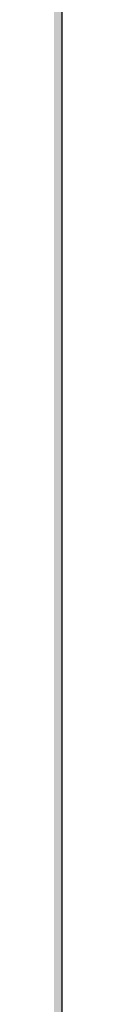
# Model space of a CAD drawing. Units: inches. Extents: x 2091 to 2899, y 967 to 2217.
# Tile 61 of 256: x 2212.1436 to 2212.1443, y 1099.9988 to 1100.1654. Entities that reach past the tile are written whole.
import ezdxf

# ---------------------------------------------------------------- set-up
doc = ezdxf.new("R2010")
doc.units = ezdxf.units.IN
doc.layers.add('A-ANNO-DIMS', color=2, linetype='Continuous', lineweight=18)
doc.layers.add('A-WALL-PATT', color=141, linetype='Continuous', lineweight=13, true_color=0xadddf7)
doc.styles.get("Standard").update_dxf_attribs({"font": 'arial.ttf'})
doc.dimstyles.new('ISO-25', dxfattribs={"dimtxt": 4, "dimasz": 4, "dimexe": 1.25, "dimexo": 0.625, "dimtad": 1, "dimdec": 0, "dimlunit": 3, "dimtxsty": 'Standard', "dimcen": 2.5, "dimadec": 0, "dimazin": 0, "dimtfac": 1, "dimtdec": 0, "dimtmove": 0, "dimatfit": 3, "dimfxl": 1, "dimarcsym": 0})

# ---------------------------------------------------------------- blocks, each defined once
blk = doc.blocks.new('*D71')
at = {"layer": 'A-ANNO-DIMS', "color": 0, "lineweight": -2, "transparency": 16777216}
for p, q in [((2212.1436, 1351.29406), (2212.1436, 969.4643)), ((2452.1436, 1351.29406), (2452.1436, 969.4643)), ((2216.1436, 970.7143), (2448.1436, 970.7143))]:
    blk.add_line(p, q, dxfattribs=at)
at = {"layer": 'A-ANNO-DIMS', "color": 0, "transparency": 16777216}
for points in [[(2216.1436, 971.38097), (2216.1436, 970.04764), (2212.1436, 970.7143)], [(2448.1436, 971.38097), (2448.1436, 970.04764), (2452.1436, 970.7143)]]:
    blk.add_solid(points, dxfattribs=at)
at = {"layer": 'Defpoints', "color": 0, "transparency": 16777216}
for p in [(2212.1436, 1351.91906), (2452.1436, 1351.91906), (2452.1436, 970.7143)]:
    blk.add_point(p, dxfattribs=at)
at = {"layer": 'A-ANNO-DIMS', "color": 0, "transparency": 16777216, "insert": (2332.1436, 973.38159), "char_height": 4, "attachment_point": 5}
blk.add_mtext('20\'-0"', dxfattribs=at)
blk = doc.blocks.new('*D75')
at = {"layer": 'A-ANNO-DIMS', "color": 0, "lineweight": -2, "transparency": 16777216}
for p, q in [((2212.1436, 1274.79406), (2212.1436, 969.4643)), ((2308.1436, 1274.79406), (2308.1436, 969.4643)), ((2216.1436, 970.7143), (2304.1436, 970.7143))]:
    blk.add_line(p, q, dxfattribs=at)
at = {"layer": 'A-ANNO-DIMS', "color": 0, "transparency": 16777216}
for points in [[(2216.1436, 971.38097), (2216.1436, 970.04764), (2212.1436, 970.7143)], [(2304.1436, 971.38097), (2304.1436, 970.04764), (2308.1436, 970.7143)]]:
    blk.add_solid(points, dxfattribs=at)
at = {"layer": 'Defpoints', "color": 0, "transparency": 16777216}
for p in [(2212.1436, 1275.41906), (2308.1436, 1275.41906), (2308.1436, 970.7143)]:
    blk.add_point(p, dxfattribs=at)
at = {"layer": 'A-ANNO-DIMS', "color": 0, "transparency": 16777216, "insert": (2260.1436, 973.38159), "char_height": 4, "attachment_point": 5}
blk.add_mtext('8\'-0"', dxfattribs=at)
blk = doc.blocks.new('*D91')
at = {"layer": 'A-ANNO-DIMS', "color": 0, "lineweight": -2, "transparency": 16777216}
for p, q in [((2211.65063, 1152.24706), (2098.31133, 1152.24706)), ((2099.56133, 1103.91906), (2099.56133, 1148.24706)), ((2211.5186, 1099.91906), (2098.31133, 1099.91906))]:
    blk.add_line(p, q, dxfattribs=at)
at = {"layer": 'A-ANNO-DIMS', "color": 0, "transparency": 16777216}
for points in [[(2098.89467, 1148.24706), (2100.228, 1148.24706), (2099.56133, 1152.24706)], [(2098.89467, 1103.91906), (2100.228, 1103.91906), (2099.56133, 1099.91906)]]:
    blk.add_solid(points, dxfattribs=at)
at = {"layer": 'Defpoints', "color": 0, "transparency": 16777216}
for p in [(2099.56133, 1152.24706), (2212.27563, 1152.24706), (2212.1436, 1099.91906)]:
    blk.add_point(p, dxfattribs=at)
at = {"layer": 'A-ANNO-DIMS', "color": 0, "transparency": 16777216, "insert": (2096.86812, 1126.08306), "char_height": 4, "attachment_point": 5, "rotation": 90}
blk.add_mtext('4\'-4 1/2"', dxfattribs=at)

msp = doc.modelspace()

# ---------------------------------------------------------------- hatches: boundary and pattern name
at = {"layer": 'A-WALL-PATT'}
h = msp.add_hatch(color=256, dxfattribs=at)
h.dxf.hatch_style = 1
h.paths.add_polyline_path([(2803.1436, 2050.91906), (2203.1436, 2050.91906), (2203.1436, 1090.91906), (2803.1436, 1090.91906)])
h.paths.add_polyline_path([(2635.79885, 1147.54046), (2674.52405, 1147.54046, 0.376086), (2678.52967, 1152.8802), (2678.52967, 1159.55647, 0.333335), (2674.52432, 1163.56185), (2674.52432, 1163.56185), (2674.52432, 1192.93439), (2635.80597, 1192.93439), (2597.08762, 1192.93439), (2597.08762, 1163.56185, 0.333335), (2593.08228, 1159.55647), (2593.08228, 1152.8802, 0.376086), (2597.08789, 1147.54046)], flags=0)
h.paths.add_polyline_path([(2436.01043, 1278.24078, 0.000483), (2435.95264, 1278.21503, -0.001328), (2435.93563, 1278.11169, -0.001711), (2436.11644, 1278.04076, 0.002185)], flags=0)
h.paths.add_polyline_path([(2794.1436, 1143.41906), (2794.1436, 1347.41906), (2543.37017, 1347.41906), (2543.37017, 1351.91906), (2794.1436, 1351.91906), (2794.1436, 1392.71355), (2793.9474, 1392.71355), (2793.9474, 1473.5369), (2794.1436, 1473.5369), (2794.1436, 1531.91906), (2650.1436, 1531.91906), (2650.1436, 1536.41906), (2794.1436, 1536.41906), (2794.1436, 1692.41906), (2609.37561, 1692.41906), (2609.37561, 1644.41906), (2604.87561, 1644.41906), (2604.87561, 1744.91906), (2609.37561, 1744.91906), (2609.37561, 1696.91906), (2794.1436, 1696.91906), (2794.1436, 1780.91906), (2609.6436, 1780.91906), (2493.87561, 1780.91906), (2493.87561, 1785.41906), (2609.6436, 1785.41906), (2794.1436, 1785.41906), (2794.1436, 1847.93882), (2793.95122, 1847.93882), (2793.95122, 1928.76217), (2794.1436, 1928.76217), (2794.1436, 1941.41906), (2614.1436, 1941.41906), (2614.1436, 1821.41906), (2609.6436, 1821.41906), (2609.6436, 1941.41906), (2392.1436, 1941.41906), (2392.1436, 1819.91906), (2387.6436, 1819.91906), (2387.6436, 1941.41906), (2212.1436, 1941.41906), (2212.1436, 1783.91906), (2392.1436, 1783.91906), (2392.1436, 1780.91906), (2212.1436, 1780.91906), (2212.1436, 1629.41906), (2387.6436, 1629.41906), (2387.6436, 1744.91906), (2392.1436, 1744.91906), (2392.1436, 1627.91906), (2317.1436, 1627.91906), (2317.1436, 1551.41906), (2317.1436, 1536.41906), (2459.38359, 1536.41906), (2459.38359, 1602.39648), (2463.88359, 1602.39648), (2463.88359, 1531.91906), (2456.6436, 1531.91906), (2456.6436, 1529.91906), (2452.1436, 1529.91906), (2452.1436, 1531.91906), (2312.6436, 1531.91906), (2312.6436, 1551.41906), (2306.1436, 1551.41906), (2306.1436, 1555.91906), (2308.1436, 1555.91906), (2308.1436, 1551.41906), (2312.6436, 1551.41906), (2312.6436, 1627.91906), (2212.1436, 1627.91906), (2212.1436, 1555.91906), (2270.1436, 1555.91906), (2270.1436, 1551.41906), (2212.1436, 1551.41906), (2212.1436, 1351.91906), (2272.1436, 1351.91906), (2272.1436, 1347.41906), (2212.1436, 1347.41906), (2212.1436, 1275.41906), (2308.1436, 1275.41906), (2308.1436, 1351.91906), (2452.1436, 1351.91906), (2452.1436, 1493.91906), (2456.6436, 1493.91906), (2456.6436, 1347.41906), (2312.6436, 1347.41906), (2312.6436, 1270.91906), (2212.1436, 1270.91906), (2212.1436, 1099.91906), (2281.23752, 1099.91906), (2282.87104, 1110.9138), (2282.00834, 1116.9966), (2278.55774, 1121.4204), (2268.20564, 1128.0562), (2272.08764, 1128.0562), (2273.81294, 1131.927), (2279.42034, 1134.6919), (2285.02784, 1135.2449), (2287.61584, 1137.4568), (2288.04714, 1138.0098), (2289.34114, 1140.7747), (2291.06654, 1139.6687), (2292.36054, 1135.2449), (2295.37984, 1136.9038), (2296.24254, 1135.7979), (2297.10524, 1133.033), (2300.12464, 1138.0098), (2303.14394, 1138.0098), (2304.43794, 1135.7979), (2303.14394, 1133.586), (2306.59464, 1134.6919), (2307.88874, 1133.033), (2310.90804, 1135.2449), (2313.92744, 1134.1389), (2315.62686, 1132.4271), (2308.32004, 1117.5496), (2290.20384, 1109.8079), (2288.90984, 1103.1721), (2289.27231, 1099.91906), (2434.91823, 1099.91906), (2431.59323, 1124.78806), (2429.93023, 1169.55306), (2430.92718, 1240.51969), (2435.65893, 1238.18613), (2437.13523, 1196.55406), (2438.79823, 1143.97306), (2442.67823, 1111.99806), (2446.55823, 1099.91906), (2794.1436, 1099.91906), (2794.1436, 1138.91906), (2548.03245, 1138.91906), (2548.03245, 1143.41906), (2548.03245, 1148.81906), (2546.66846, 1148.03156), (2528.68569, 1179.17862, 0.256256), (2512.03245, 1148.81906), (2512.03245, 1143.41906), (2512.03245, 1138.91906), (2507.53245, 1138.91906), (2507.53245, 1143.41906), (2507.53245, 1148.81906, 0.256256), (2490.8792, 1179.17862), (2472.89644, 1148.03156), (2471.53245, 1148.81906), (2471.53245, 1143.41906), (2467.03245, 1143.41906), (2467.03245, 1269.94579, 0.039061), (2460.90999, 1273.58006), (2467.03245, 1273.58006), (2467.03245, 1286.32536, 0.014511), (2465.21619, 1286.76191), (2467.03245, 1287.05258), (2467.03245, 1323.41906), (2471.53245, 1323.41906), (2471.53245, 1148.81906), (2489.53245, 1179.99597), (2490.89644, 1179.20847), (2490.8792, 1179.17862, -0.256256), (2507.53245, 1148.81906), (2507.53245, 1143.41906), (2512.03245, 1143.41906), (2512.03245, 1148.81906, -0.256256), (2528.68569, 1179.17862), (2528.66846, 1179.20847), (2530.03245, 1179.99597), (2548.03245, 1148.81906), (2548.03245, 1143.41906)], flags=16)
h.paths.add_polyline_path([(2607.76855, 1200.94508), (2607.76855, 1265.03063), (2597.08762, 1281.05201), (2619.78459, 1281.05201), (2627.79528, 1337.12686), (2635.79885, 1337.12686), (2643.81666, 1337.12686), (2651.82736, 1281.05201), (2674.52432, 1281.05201), (2663.8434, 1265.03063), (2663.8434, 1200.94508), (2635.80597, 1200.94508)], flags=0)
edge = h.paths.add_edge_path(flags=0)
edge.add_ellipse((13303.89622, 1272.99872), major_axis=(-10595.31304, 0), ratio=0.84230387009, start_angle=0.628237219, end_angle=0.6465541, ccw=False)
edge.add_ellipse((2711.70045, 1156.85268), major_axis=(2.21977, 0), ratio=0.8423039, start_angle=111.53524, end_angle=180.62824, ccw=False)
edge.add_ellipse((13303.15629, 1272.99872), major_axis=(-10593.02631, 0), ratio=0.84230386954, start_angle=0.528271472, end_angle=0.646554097, ccw=False)
edge.add_line((2710.7646, 1175.3333), (2710.12999, 1175.3333))
edge.add_ellipse((2710.12999, 1176.57978), major_axis=(1.47985, 0), ratio=0.8423039, start_angle=180, end_angle=270, ccw=False)
edge.add_line((2708.65014, 1176.57978), (2708.65014, 1200.78291))
edge.add_ellipse((2710.12999, 1200.78291), major_axis=(1.47985, 0), ratio=0.8423039, start_angle=90, end_angle=180, ccw=False)
edge.add_line((2710.12999, 1202.02939), (2710.46508, 1202.02939))
edge.add_ellipse((13303.15629, 1272.99872), major_axis=(-10593.02631, 0), ratio=0.84230386954, start_angle=-0.090229089, end_angle=0.383866779, ccw=False)
edge.add_ellipse((2710.12999, 1290.92703), major_axis=(-1.47985, 0), ratio=0.8423039, start_angle=0, end_angle=90, ccw=False)
edge.add_line((2708.65014, 1290.92703), (2708.65014, 1315.13017))
edge.add_ellipse((2710.12999, 1315.13017), major_axis=(-1.47985, 0), ratio=0.8423039, start_angle=-90, end_angle=0, ccw=False)
edge.add_line((2710.12999, 1316.37665), (2710.70631, 1316.37665))
edge.add_ellipse((3238.40172, 1296.28957), major_axis=(528.234, 0), ratio=0.84230387, start_angle=176.3495724, end_angle=177.8200497, ccw=False)
edge.add_ellipse((2775.06304, 1071.4507), major_axis=(313.30776, 0), ratio=0.84230387, start_angle=102.1259656, end_angle=103.780529, ccw=False)
edge.add_ellipse((2775.06304, 1078.3057), major_axis=(-305.30289, 0), ratio=0.84230387, start_angle=-79.790461, end_angle=-77.5553727, ccw=False)
edge.add_ellipse((2695.14177, 1541.97538), major_axis=(-250.96022, 0), ratio=0.84230387, start_angle=99.256566, end_angle=102.5549326)
edge.add_line((2741.41033, 1334.21426), (2747.13255, 1337.37848))
edge.add_ellipse((2747.53862, 1336.85748), major_axis=(-0.73992, 0), ratio=0.842304, start_angle=270, end_angle=307.93313, ccw=False)
edge.add_ellipse((2747.53862, 1336.85748), major_axis=(-0.73992, 0), ratio=0.842304, start_angle=232.06687, end_angle=270, ccw=False)
edge.add_line((2747.94469, 1337.37848), (2753.66691, 1334.21426))
edge.add_ellipse((2799.93547, 1541.97538), major_axis=(250.96022, 0), ratio=0.84230387, start_angle=257.4450674, end_angle=260.743434)
edge.add_ellipse((2720.01419, 1078.3057), major_axis=(305.30289, 0), ratio=0.84230387, start_angle=77.5553727, end_angle=79.790461, ccw=False)
edge.add_ellipse((2720.01419, 1071.4507), major_axis=(-313.30776, 0), ratio=0.84230387, start_angle=256.219471, end_angle=257.8740344, ccw=False)
edge.add_ellipse((2256.67551, 1296.28957), major_axis=(-528.234, 0), ratio=0.84230387, start_angle=182.1799503, end_angle=183.6504276, ccw=False)
edge.add_line((2784.37092, 1316.37665), (2784.94725, 1316.37665))
edge.add_ellipse((2784.94725, 1315.13017), major_axis=(1.47985, 0), ratio=0.8423039, start_angle=0, end_angle=90, ccw=False)
edge.add_line((2786.42709, 1315.13017), (2786.42709, 1290.92703))
edge.add_ellipse((2784.94725, 1290.92703), major_axis=(1.47985, 0), ratio=0.8423039, start_angle=270, end_angle=360, ccw=False)
edge.add_ellipse((-7808.07906, 1272.99872), major_axis=(10593.02631, 0), ratio=0.84230386954, start_angle=-0.383866779, end_angle=0.090229089, ccw=False)
edge.add_line((2784.61216, 1202.02939), (2784.94725, 1202.02939))
edge.add_ellipse((2784.94725, 1200.78291), major_axis=(1.47985, 0), ratio=0.8423039, start_angle=0, end_angle=90, ccw=False)
edge.add_line((2786.42709, 1200.78291), (2786.42709, 1176.57978))
edge.add_ellipse((2784.94725, 1176.57978), major_axis=(-1.47985, 0), ratio=0.8423039, start_angle=90, end_angle=180, ccw=False)
edge.add_line((2784.94725, 1175.3333), (2784.31264, 1175.3333))
edge.add_ellipse((-7808.07906, 1272.99872), major_axis=(10593.02631, 0), ratio=0.84230386954, start_angle=-0.618643196, end_angle=-0.528271472, ccw=False)
edge.add_ellipse((2783.37678, 1156.85268), major_axis=(-2.21977, 0), ratio=0.8423039, start_angle=179.37176, end_angle=248.46476, ccw=False)
edge.add_ellipse((-7808.81898, 1272.99872), major_axis=(-10595.31304, 0), ratio=0.84230386576, start_angle=179.353445923, end_angle=179.371762803, ccw=False)
edge.add_ellipse((2780.2973, 1153.50079), major_axis=(-5.24643, 0), ratio=0.8423039, start_angle=90, end_angle=179.35345, ccw=False)
edge.add_line((2780.2973, 1149.08171), (2714.77993, 1149.08171))
edge.add_ellipse((2714.77993, 1153.50079), major_axis=(5.24643, 0), ratio=0.8423039, start_angle=180.64655, end_angle=270, ccw=False)
edge = h.paths.add_edge_path(flags=0)
edge.add_line((2718.18737, 1151.00783), (2718.18737, 1170.47236))
edge.add_ellipse((2721.14706, 1170.47236), major_axis=(-2.95969, 0), ratio=0.8423039, start_angle=-90, end_angle=0, ccw=False)
edge.add_line((2721.14706, 1172.96532), (2773.93017, 1172.96532))
edge.add_ellipse((2773.93017, 1170.47236), major_axis=(-2.95969, 0), ratio=0.8423039, start_angle=180, end_angle=270, ccw=False)
edge.add_line((2776.88987, 1170.47236), (2776.88987, 1151.00783))
edge.add_line((2776.88987, 1151.00783), (2718.18737, 1151.00783))
edge = h.paths.add_edge_path(flags=0)
edge.add_line((2718.18737, 1180.23415), (2718.18737, 1199.05783))
edge.add_ellipse((2747.53862, 1320.39864), major_axis=(147.01792, 0), ratio=0.84230387, start_angle=256.4018653, end_angle=283.5981347)
edge.add_line((2776.88987, 1199.05783), (2776.88987, 1180.23415))
edge.add_ellipse((2747.53862, 1301.57496), major_axis=(147.01792, 0), ratio=0.84230387, start_angle=256.4018653, end_angle=283.5981347, ccw=False)
edge = h.paths.add_edge_path(flags=0)
edge.add_ellipse((13303.15629, 1272.99872), major_axis=(-10591.54646, 0), ratio=0.84230386955, start_angle=0.055594314, end_angle=0.377764194, ccw=False)
edge.add_line((2711.61686, 1262.72171), (2715.66741, 1249.4954))
edge.add_ellipse((6413.89196, 1241.69192), major_axis=(-3698.23616, 0), ratio=0.8423038695, start_angle=-0.12089737, end_angle=0.36407635)
edge.add_line((2715.76104, 1218.19245), (2711.93431, 1203.16736))
edge = h.paths.add_edge_path(flags=0)
edge.add_line((2718.18737, 1251.07457), (2716.00249, 1267.45044))
edge.add_ellipse((2742.15117, 1202.18954), major_axis=(81.77258, 0), ratio=0.84230387, start_angle=94.277421, end_angle=111.8349538, ccw=False)
edge.add_line((2737.00975, 1270.93063), (2758.06748, 1270.93063))
edge.add_ellipse((2752.92606, 1202.18954), major_axis=(81.77258, 0), ratio=0.84230387, start_angle=68.1650462, end_angle=85.722579, ccw=False)
edge.add_line((2779.07475, 1267.45044), (2776.88987, 1251.07457))
edge.add_ellipse((2750.33806, 1187.88536), major_axis=(79.57966, 0), ratio=0.84230387, start_angle=67.2080851, end_angle=85.1299304)
edge.add_line((2756.03466, 1254.74366), (2739.04258, 1254.74366))
edge.add_ellipse((2744.73917, 1187.88536), major_axis=(79.57966, 0), ratio=0.84230387, start_angle=94.8700696, end_angle=112.7919149)
edge = h.paths.add_edge_path(flags=0)
edge.add_line((2783.14293, 1203.16736), (2779.31619, 1218.19245))
edge.add_ellipse((-918.81473, 1241.69192), major_axis=(3698.23616, 0), ratio=0.8423038695, start_angle=-0.36407635, end_angle=0.12089737)
edge.add_line((2779.40983, 1249.4954), (2783.46037, 1262.72171))
edge.add_ellipse((-7808.07906, 1272.99872), major_axis=(-10591.54646, 0), ratio=0.84230386954, start_angle=179.622235806, end_angle=179.944405687, ccw=False)
edge = h.paths.add_edge_path(flags=0)
edge.add_ellipse((2734.20089, 1286.69044), major_axis=(-0.35661, 6.34008), ratio=0.6038336, start_angle=89.002014, end_angle=253.657408, ccw=False)
edge.add_line((2730.369, 1286.54181), (2730.369, 1301.35198))
edge.add_line((2730.369, 1301.35198), (2735.91331, 1305.2148))
edge.add_ellipse((2736.38492, 1304.73456), major_axis=(0.73992, 0), ratio=0.842304, start_angle=90, end_angle=134.48021, ccw=False)
edge.add_line((2736.38492, 1305.3578), (2738.03278, 1305.3578))
edge.add_line((2738.03278, 1305.3578), (2738.03278, 1307.70793))
edge.add_ellipse((2794.20164, 1307.70793), major_axis=(56.16886, 0), ratio=0.84230387, start_angle=150.56143, end_angle=180, ccw=False)
edge.add_ellipse((2700.87559, 1307.70793), major_axis=(-56.16886, 0), ratio=0.84230387, start_angle=180, end_angle=209.43857, ccw=False)
edge.add_line((2757.04445, 1307.70793), (2757.04445, 1305.3578))
edge.add_line((2757.04445, 1305.3578), (2758.69232, 1305.3578))
edge.add_ellipse((2758.69232, 1304.73456), major_axis=(-0.73992, 0), ratio=0.842304, start_angle=225.51979, end_angle=270, ccw=False)
edge.add_line((2759.16392, 1305.2148), (2764.70823, 1301.35198))
edge.add_line((2764.70823, 1301.35198), (2764.70823, 1286.54181))
edge.add_ellipse((2760.87634, 1286.69044), major_axis=(0.35661, 6.34008), ratio=0.6038336, start_angle=106.342592, end_angle=270.997986, ccw=False)
edge.add_line((2757.04445, 1285.79709), (2757.04445, 1307.70793))
edge.add_ellipse((2700.87559, 1307.70793), major_axis=(-56.16886, 0), ratio=0.84230387, start_angle=180, end_angle=209.43857)
edge.add_ellipse((2794.20164, 1307.70793), major_axis=(56.16886, 0), ratio=0.84230387, start_angle=150.56143, end_angle=180)
edge.add_line((2738.03278, 1307.70793), (2738.03278, 1285.79709))
h.paths.add_polyline_path([(2417.81227, 1104.4497), (2413.49227, 1102.5297), (2410.61227, 1103.9697), (2409.17227, 1106.3697), (2407.25227, 1107.3297), (2406.29227, 1109.7297), (2405.33227, 1114.0497), (2405.33227, 1117.8897), (2406.29227, 1120.1297), (2407.25227, 1119.8097), (2408.84832, 1118.32766), (2410.17395, 1119.42417), (2410.21127, 1120.4057), (2411.04073, 1121.41905), (2410.69927, 1119.8587), (2410.17395, 1119.42417), (2410.08845, 1117.17611), (2411.13284, 1116.20632), (2413.97227, 1119.3297), (2416.85227, 1120.7697), (2416.86972, 1120.79878), (2417.03507, 1119.40512), (2417.89621, 1118.14338), (2418.29227, 1118.3697), (2419.54445, 1120.03927), (2419.36092, 1118.38749), (2419.03211, 1119.35615), (2418.39894, 1118.51193), (2419.25227, 1114.5297), (2418.79409, 1107.19879)], flags=0)
h.paths.add_polyline_path([(2508.87017, 1347.41906), (2508.37017, 1347.41906), (2508.37017, 1351.91906), (2508.87017, 1351.91906)], flags=0)
h.paths.add_polyline_path([(2473.37017, 1347.41906), (2472.37017, 1347.41906), (2467.87017, 1347.41906), (2467.87017, 1455.41906), (2472.37017, 1455.41906), (2472.37017, 1352.41906), (2473.37017, 1352.41906)], flags=0)
h.paths.add_polyline_path([(2352.10624, 1217.4462), (2349.22624, 1218.8862), (2347.78624, 1221.2862), (2345.86624, 1222.2462), (2344.90624, 1224.6462), (2343.94624, 1228.9662), (2343.94624, 1232.8062), (2344.90624, 1235.0462), (2345.86624, 1234.7262), (2347.46229, 1233.24415), (2348.78792, 1234.34066), (2348.82524, 1235.3222), (2349.6547, 1236.33555), (2349.31324, 1234.7752), (2348.78792, 1234.34066), (2348.70242, 1232.0926), (2349.74681, 1231.12282), (2352.58624, 1234.2462), (2355.46624, 1235.6862), (2355.48369, 1235.71528), (2355.64904, 1234.32161), (2356.51018, 1233.05988), (2356.90624, 1233.2862), (2358.15842, 1234.95576), (2357.97489, 1233.30398), (2357.64608, 1234.27264), (2357.01291, 1233.42842), (2357.86624, 1229.4462), (2357.40806, 1222.11529), (2356.42624, 1219.3662)], flags=0)
h.paths.add_polyline_path([(2348.2968, 1112.22442), (2347.0138, 1112.31042), (2345.5298, 1114.12742), (2345.7318, 1115.85842), (2346.8118, 1116.98242), (2346.8118, 1114.64642), (2345.8668, 1114.21442), (2346.8798, 1114.30042)], flags=0)
h.paths.add_polyline_path([(2347.0138, 1110.92642), (2346.2718, 1110.49342), (2346.6098, 1111.18642)], flags=0)
h.paths.add_polyline_path([(2345.8668, 1118.19442), (2345.5298, 1117.32942), (2343.7078, 1118.02142), (2344.3828, 1118.62642)], flags=0)
h.paths.add_polyline_path([(2346.6768, 1109.28242), (2346.0698, 1108.07142), (2345.8668, 1110.06142)], flags=0)
h.paths.add_polyline_path([(2345.0568, 1119.75142), (2343.6398, 1119.75142), (2343.9778, 1121.13542)], flags=0)
h.paths.add_polyline_path([(2345.2598, 1116.55042), (2345.1248, 1115.85842), (2344.9218, 1115.68542), (2344.7198, 1116.37742)], flags=0)
h.paths.add_polyline_path([(2345.6648, 1112.31042), (2345.4618, 1111.53242), (2344.0448, 1111.96442), (2344.6518, 1112.57042)], flags=0)
h.paths.add_polyline_path([(2345.1918, 1113.34942), (2344.4498, 1113.86842), (2344.7198, 1114.38742)], flags=0)
h.paths.add_polyline_path([(2344.6518, 1116.80942), (2344.1798, 1115.68542), (2344.6518, 1115.33942), (2343.9098, 1114.90642), (2343.0328, 1115.94442), (2343.6398, 1116.46342)], flags=0)
h.paths.add_polyline_path([(2345.8668, 1106.68642), (2344.9898, 1105.56242), (2344.5168, 1106.60042)], flags=0)
h.paths.add_polyline_path([(2344.8548, 1110.06142), (2344.5168, 1109.28242), (2344.1128, 1109.71542)], flags=0)
h.paths.add_polyline_path([(2344.0448, 1113.52242), (2343.4378, 1113.08942), (2342.7628, 1113.95442)], flags=0)
h.paths.add_polyline_path([(2344.3148, 1111.01242), (2342.9648, 1110.32042), (2342.9648, 1111.09942)], flags=0)
h.paths.add_polyline_path([(2345.1248, 1104.69742), (2344.5848, 1103.74542), (2344.4498, 1104.26442)], flags=0)
h.paths.add_polyline_path([(2342.8298, 1121.22242), (2341.7498, 1120.53042), (2340.5358, 1121.04942), (2340.1308, 1121.82842), (2340.6708, 1122.95242), (2341.1428, 1121.82842), (2341.6148, 1122.00142)], flags=0)
h.paths.add_polyline_path([(2342.9648, 1119.75142), (2343.0328, 1118.45342), (2342.0878, 1118.02142), (2342.0198, 1119.49142)], flags=0)
h.paths.add_polyline_path([(2342.6948, 1116.89642), (2341.9528, 1116.63642), (2342.0198, 1117.32942)], flags=0)
h.paths.add_polyline_path([(2343.0328, 1112.22442), (2342.0198, 1111.79142), (2341.5478, 1112.22442), (2342.3578, 1113.34942)], flags=0)
h.paths.add_polyline_path([(2343.7748, 1104.43742), (2342.6278, 1102.88042), (2342.6948, 1104.61042), (2343.4378, 1105.12942)], flags=0)
h.paths.add_polyline_path([(2342.0198, 1115.07942), (2340.8058, 1115.51242), (2340.9408, 1116.37742)], flags=0)
h.paths.add_polyline_path([(2341.4808, 1120.09742), (2341.4808, 1119.40542), (2341.0758, 1119.57842), (2341.1428, 1120.09742)], flags=0)
h.paths.add_polyline_path([(2341.8178, 1114.47342), (2340.9408, 1113.08942), (2340.8058, 1114.56042)], flags=0)
h.paths.add_polyline_path([(2341.1428, 1118.54042), (2340.9408, 1116.98242), (2339.0508, 1117.67542), (2339.0508, 1118.62642)], flags=0)
h.paths.add_polyline_path([(2342.6948, 1101.66842), (2341.9528, 1101.84142), (2342.5598, 1102.36142)], flags=0)
h.paths.add_polyline_path([(2340.3328, 1119.66542), (2338.4438, 1119.57842), (2337.9038, 1120.35742), (2339.6578, 1120.61642)], flags=0)
h.paths.add_polyline_path([(2340.3328, 1115.33942), (2340.0628, 1113.69542), (2339.3878, 1115.33942)], flags=0)
h.paths.add_polyline_path([(2341.8178, 1103.83142), (2341.5478, 1102.88042), (2341.1428, 1103.65842)], flags=0)
h.paths.add_polyline_path([(2339.0508, 1122.86642), (2337.2958, 1121.82842), (2337.0938, 1123.12542), (2337.7688, 1123.81842)], flags=0)
h.paths.add_polyline_path([(2339.1178, 1121.74142), (2338.8478, 1121.22242), (2338.1738, 1121.04942), (2338.3758, 1121.56842)], flags=0)
h.paths.add_polyline_path([(2339.1858, 1119.31942), (2338.6458, 1118.71342), (2338.2408, 1118.10742), (2338.2408, 1118.88642)], flags=0)
h.paths.add_polyline_path([(2341.1428, 1101.92842), (2340.6028, 1101.23642), (2340.0628, 1101.84142), (2340.6028, 1102.36142)], flags=0)
h.paths.add_polyline_path([(2337.6338, 1117.76142), (2336.6208, 1118.28042), (2337.2958, 1118.97242)], flags=0)
h.paths.add_polyline_path([(2336.8238, 1119.57842), (2334.7988, 1118.97242), (2335.2038, 1120.35742), (2336.5538, 1120.87642)], flags=0)
h.paths.add_polyline_path([(2339.1178, 1100.45742), (2337.3638, 1100.54342), (2336.7558, 1101.23642)], flags=0)
h.paths.add_polyline_path([(2336.3508, 1122.43342), (2336.0138, 1121.91442), (2334.9338, 1122.43342), (2334.5288, 1123.47142), (2335.7438, 1122.77942)], flags=0)
h.paths.add_polyline_path([(2334.7318, 1120.87642), (2334.2588, 1120.35742), (2334.0568, 1120.78942), (2334.5968, 1121.30842)], flags=0)
h.paths.add_polyline_path([(2334.4618, 1122.17442), (2332.5718, 1121.30842), (2331.3568, 1122.17442), (2332.0998, 1122.86642)], flags=0)
h.paths.add_polyline_path([(2334.2588, 1118.54042), (2333.3818, 1118.45342), (2333.6518, 1119.31942)], flags=0)
h.paths.add_polyline_path([(2335.5418, 1102.27442), (2334.1918, 1102.62042), (2335.2718, 1103.31242)], flags=0)
h.paths.add_polyline_path([(2332.7068, 1119.66542), (2331.6948, 1120.44342), (2332.5048, 1120.78942)], flags=0)
h.paths.add_polyline_path([(2334.7318, 1101.14942), (2333.5168, 1101.58242), (2333.9888, 1101.75542)], flags=0)
h.paths.add_polyline_path([(2332.6398, 1116.63642), (2331.0868, 1116.29042), (2331.9648, 1118.19442)], flags=0)
h.paths.add_polyline_path([(2330.7498, 1121.56842), (2330.2768, 1120.27042), (2328.5228, 1119.31942), (2328.9948, 1121.04942)], flags=0)
h.paths.add_polyline_path([(2330.7498, 1118.62642), (2330.0078, 1117.50242), (2329.8728, 1118.02142)], flags=0)
h.paths.add_polyline_path([(2332.0998, 1102.36142), (2330.5468, 1102.01442), (2331.6948, 1102.96642)], flags=0)
h.paths.add_polyline_path([(2329.5348, 1113.60842), (2329.0628, 1112.31042), (2328.5898, 1113.34942)], flags=0)
h.paths.add_polyline_path([(2328.3878, 1117.84842), (2327.5098, 1116.55042), (2327.1728, 1117.76142)], flags=0)
h.paths.add_polyline_path([(2329.7378, 1106.51342), (2329.5348, 1105.30242), (2328.2528, 1106.08142)], flags=0)
h.paths.add_polyline_path([(2328.6578, 1114.38742), (2328.0498, 1114.12742), (2328.3198, 1114.90642)], flags=0)
h.paths.add_polyline_path([(2328.3198, 1112.22442), (2327.1058, 1112.13742), (2326.7008, 1112.65642)], flags=0)
h.paths.add_polyline_path([(2326.9028, 1115.25242), (2326.7008, 1114.12742), (2325.2158, 1113.60842), (2326.0928, 1115.33942)], flags=0)
h.paths.add_polyline_path([(2326.6328, 1108.33042), (2326.0928, 1107.37942), (2325.8908, 1108.50342), (2326.4978, 1109.10942)], flags=0)
h.paths.add_polyline_path([(2615.1436, 1531.91906), (2609.6436, 1531.91906), (2609.6436, 1620.41906), (2614.1436, 1620.41906), (2614.1436, 1536.41906), (2615.1436, 1536.41906)], flags=0)
h.paths.add_polyline_path([(2545.1436, 1563.41906), (2464.1436, 1563.41906), (2464.1436, 1632.41906), (2509.1436, 1632.41906), (2509.1436, 1627.91906), (2509.1436, 1603.91906), (2468.6436, 1603.91906), (2468.6436, 1567.91906), (2540.6436, 1567.91906), (2540.6436, 1591.91906), (2545.1436, 1591.91906)], flags=0)
h.paths.add_polyline_path([(2388.96905, 1549.98573), (2357.43418, 1549.98573), (2357.43418, 1623.36078), (2399.36278, 1623.36078), (2435.68947, 1623.36078), (2435.59255, 1602.55927), (2435.59255, 1602.39648), (2388.96905, 1602.39648)], flags=0)
h.paths.add_polyline_path([(2388.88063, 1555.80915), (2374.90443, 1555.80915), (2374.90443, 1600.57156), (2374.90443, 1615.45765), (2406.35088, 1615.45765), (2406.35088, 1618.93943), (2412.17429, 1615.45765), (2406.35088, 1611.97586), (2406.35088, 1615.45765), (2388.88063, 1615.45765)], flags=0)
h.paths.add_polyline_path([(2568.87561, 1644.41906), (2453.37561, 1644.41906), (2453.37561, 1785.41906), (2457.87561, 1785.41906), (2457.87561, 1648.91906), (2568.87561, 1648.91906)], flags=0)
h.paths.add_polyline_path([(2212.1436, 1945.91906), (2212.1436, 2041.91906), (2794.1436, 2041.91906), (2794.1436, 1945.91906)], flags=16)
h.paths.add_polyline_path([(2271.08273, 1964.31724), (2776.85297, 1964.31724), (2776.85297, 2037.16962), (2271.08273, 2037.16962)], flags=8)
h.paths.add_polyline_path([(2380.64929, 1536.82414), (2461.04081, 1536.82414), (2461.04081, 1554.65259), (2380.64929, 1554.65259)], flags=8)
h.paths.add_polyline_path([(2240.75571, 1609.72545), (2309.18583, 1609.72545), (2309.18583, 1617.6982), (2240.75571, 1617.6982)], flags=8)
h.paths.add_polyline_path([(2212.67726, 1313.5041), (2282.59152, 1313.5041), (2282.59152, 1322.74524), (2212.67726, 1322.74524)], flags=8)
h.paths.add_polyline_path([(2457.11198, 1114.77857), (2558.48158, 1114.77857), (2558.48158, 1142.21968), (2457.11198, 1142.21968)], flags=8)
h.paths.add_polyline_path([(2473.44234, 1273.01007), (2604.64123, 1273.01007), (2604.64123, 1318.34693), (2473.44234, 1318.34693)], flags=8)
h.paths.add_polyline_path([(2638.8763, 1626.97743), (2684.25037, 1627.97674), (2684.03848, 1637.59749), (2638.66442, 1636.59819)], flags=8)
h.paths.add_polyline_path([(2537.59055, 1453.79345), (2628.38955, 1453.79345), (2628.38955, 1475.34481), (2537.59055, 1475.34481)], flags=8)
h.paths.add_polyline_path([(2504.13764, 1714.6324), (2554.64719, 1714.6324), (2554.64719, 1730.23771), (2504.13764, 1730.23771)], flags=8)
h.paths.add_polyline_path([(2487.50118, 1575.65187), (2535.09712, 1575.65187), (2535.09712, 1598.37765), (2487.50118, 1598.37765)], flags=8)
h.paths.add_polyline_path([(2709.0994, 1735.71028), (2740.0166, 1735.71028), (2740.0166, 1749.93764), (2709.0994, 1749.93764)], flags=8)
h.paths.add_polyline_path([(2442.43842, 1792.17166), (2564.72884, 1792.17166), (2564.72884, 1842.00016), (2442.43842, 1842.00016)], flags=8)
h.paths.add_polyline_path([(2655.8158, 1809.64408), (2789.52014, 1806.6938), (2790.08498, 1832.29164), (2656.38064, 1835.24192)], flags=8)
h.paths.add_polyline_path([(2234.8427, 1797.72014), (2368.59285, 1794.76885), (2369.16072, 1820.50413), (2235.41056, 1823.45542)], flags=8)
h.paths.add_polyline_path([(2245.13847, 1644.00633), (2398.42773, 1640.6239), (2398.99484, 1666.32482), (2245.70557, 1669.70725)], flags=8)
h.paths.add_polyline_path([(2306.14285, 1431.16852), (2413.76831, 1428.79369), (2414.33315, 1454.39153), (2306.70768, 1456.76636)], flags=8)
h.paths.add_polyline_path([(2306.83458, 1458.23314), (2393.38048, 1456.32345), (2393.93281, 1481.35436), (2307.38691, 1483.26405)], flags=8)

# ---------------------------------------------------------------- dimensions: what is measured, and where the dimension line sits
at = {"layer": 'A-ANNO-DIMS'}
for base, p1, p2, picture, middle in [((2452.1436, 970.7143), (2212.1436, 1351.91906), (2452.1436, 1351.91906), '*D71', (2332.1436, 973.38159)), ((2308.1436, 970.7143), (2212.1436, 1275.41906), (2308.1436, 1275.41906), '*D75', (2260.1436, 973.38159))]:
    dim = msp.add_linear_dim(base=base, p1=p1, p2=p2, dimstyle='ISO-25', override={"dimdec": 1, "dimlfac": 1, "dimrnd": 0, "dimzin": 1, "dimdsep": 46, "dimlunit": 4, "dimfrac": 2}, dxfattribs=at)
    dim.commit()
    dim.dimension.update_dxf_attribs({"geometry": picture, "text_midpoint": middle})
dim = msp.add_linear_dim(base=(2099.56133, 1152.24706), p1=(2212.1436, 1099.91906), p2=(2212.27563, 1152.24706), angle=90, dimstyle='ISO-25', override={"dimdec": 1, "dimlfac": 1, "dimrnd": 0, "dimzin": 1, "dimdsep": 46, "dimlunit": 4, "dimfrac": 2}, dxfattribs=at)
dim.commit()
dim.dimension.update_dxf_attribs({"geometry": '*D91', "text_midpoint": (2096.86812, 1126.08306)})

doc.saveas('drawing.dxf')
